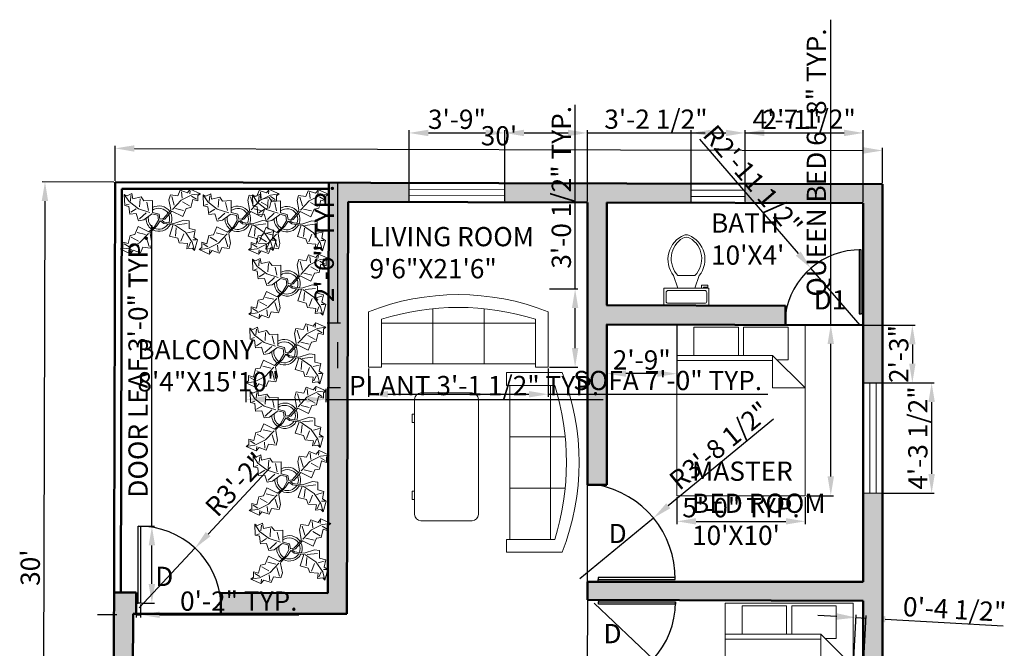
# Model space of a CAD drawing. Units: inches. Extents: x 16989 to 17950, y 7982 to 8536.
# Tile 5 of 5: x 17489 to 17950, y 8242 to 8536. Entities that reach past the tile are written whole.
import ezdxf

# ---------------------------------------------------------------- set-up
doc = ezdxf.new("R2010")
doc.units = ezdxf.units.IN
for name, color, linetype, lineweight in [('A-ANNO-DIMS', 2, 'Continuous', 18), ('A-ANNO-IDEN', 7, 'Continuous', 18), ('A-AREA-IDEN', 7, 'Continuous', 25), ('A-DOOR', 3, 'Continuous', 25), ('A-FLOR-FIXT', 9, 'Continuous', 18), ('A-FURN', 8, 'Continuous', 18), ('A-GLAZ', 4, 'Continuous', 18), ('A-WALL', 7, 'Continuous', 50), ('L-PLNT', 94, 'Continuous', 13)]:
    doc.layers.add(name, color=color, linetype=linetype, lineweight=lineweight)
doc.layers.add('A-WALL-PATT', color=177, linetype='Continuous', lineweight=13, true_color=0x293189)
doc.styles.get("Standard").update_dxf_attribs({"font": 'arial.ttf'})
doc.dimstyles.new('ISO-25', dxfattribs={"dimtxt": 9, "dimasz": 9, "dimexe": 1.25, "dimexo": 0.625, "dimtad": 1, "dimdec": 1, "dimrnd": 9, "dimlunit": 3, "dimtxsty": 'Standard', "dimcen": 2.5, "dimadec": 0, "dimazin": 0, "dimtfac": 1, "dimtdec": 1, "dimtmove": 0, "dimatfit": 3, "dimfxl": 1, "dimarcsym": 0})

# ---------------------------------------------------------------- blocks, each defined once
blk = doc.blocks.new('*D10')
at = {"layer": 'A-ANNO-DIMS', "color": 0, "lineweight": -2, "transparency": 16777216}
for p, q in [((17533.26, 8460.26), (17499.84, 8460.35)), ((17501.06, 8451.35), (17500.13, 8108.37)), ((17532.27, 8099.28), (17498.85, 8099.37))]:
    blk.add_line(p, q, dxfattribs=at)
at = {"layer": 'A-ANNO-DIMS', "color": 0, "transparency": 16777216}
for points in [[(17499.56, 8451.35), (17502.56, 8451.34), (17501.09, 8460.35)], [(17498.63, 8108.37), (17501.63, 8108.36), (17500.1, 8099.37)]]:
    blk.add_solid(points, dxfattribs=at)
at = {"layer": 'Defpoints', "color": 0, "transparency": 16777216}
for p in [(17533.88, 8460.26), (17500.1, 8099.37), (17532.9, 8099.28)]:
    blk.add_point(p, dxfattribs=at)
at = {"layer": 'A-ANNO-DIMS', "color": 0, "transparency": 16777216, "insert": (17495.37, 8279.87), "char_height": 9, "attachment_point": 5, "rotation": 89.8438}
blk.add_mtext("30'", dxfattribs=at)
blk = doc.blocks.new('*D11')
at = {"layer": 'A-ANNO-DIMS', "color": 0, "lineweight": -2, "transparency": 16777216}
for p, q in [((17533.88, 8460.88), (17533.93, 8477.23)), ((17542.93, 8475.95), (17883.94, 8475.02)), ((17892.9, 8459.9), (17892.94, 8476.25))]:
    blk.add_line(p, q, dxfattribs=at)
at = {"layer": 'A-ANNO-DIMS', "color": 0, "transparency": 16777216}
for points in [[(17542.93, 8477.45), (17542.92, 8474.45), (17533.93, 8475.98)], [(17883.95, 8476.52), (17883.94, 8473.52), (17892.94, 8475)]]:
    blk.add_solid(points, dxfattribs=at)
at = {"layer": 'Defpoints', "color": 0, "transparency": 16777216}
for p in [(17892.94, 8475), (17533.88, 8460.26), (17892.9, 8459.28)]:
    blk.add_point(p, dxfattribs=at)
at = {"layer": 'A-ANNO-DIMS', "color": 0, "transparency": 16777216, "insert": (17713.45, 8480.71), "char_height": 9, "attachment_point": 5, "rotation": 359.8438}
blk.add_mtext("30'", dxfattribs=at)
blk = doc.blocks.new('Plant - Rubber or Philodendron')
for p, q in [((13.3837, 12.301), (14.68, 13.9039)), ((14.68, 13.9039), (19.3848, 11.8146)), ((-16.2005, 11.4774), (-13.9899, 8.1064)), ((-16.2005, 11.4774), (-14.8639, 10.7964)), ((-16.0159, 6.3329), (-16.2005, 11.4774)), ((-14.8639, 10.7964), (-12.6195, 11.8975)), ((-13.3174, 8.325), (-13.0735, 11.0065)), ((-12.6195, 11.8975), (-12.1909, 9.4345)), ((-12.1909, 9.4345), (-8.3829, 10.3)), ((-8.8369, 9.409), (-9.0894, 5.6095)), ((-8.3829, 10.3), (-7.0549, 8.501)), ((4.6914, 8.8812), (5.3859, 11.2828)), ((5.3859, 11.2828), (8.8871, 10.7908)), ((5.9878, 10.4842), (7.1971, 6.3869)), ((8.8871, 10.7908), (9.9809, 13.4933)), ((9.9809, 13.4933), (13.3837, 12.301)), ((15.3859, 11.3055), (10.3916, 8.7942)), ((10.5828, 12.6946), (10.8893, 9.7953)), ((14.5816, 13.2037), (14.3848, 11.8033)), ((15.2875, 10.6053), (17.5907, 9.2105)), ((19.3848, 11.8146), (15.3859, 11.3055)), ((19.3848, 11.8146), (18.1868, 10.9119)), ((18.1868, 10.9119), (18.1925, 8.4119)), ((-14.0069, 5.8704), (-16.0159, 6.3329)), ((-15.3434, 6.5514), (-13.9984, 6.9884)), ((-13.5868, 2.2894), (-14.0069, 5.8704)), ((-13.9899, 8.1064), (-9.5434, 4.7185)), ((-13.1329, 3.1804), (-10.6614, 4.727)), ((-9.5434, 4.7185), (-4.1917, 2.9888)), ((-7.0549, 8.501), (-3.0284, 8.6941)), ((-4.8529, 4.012), (-5.7184, 7.82)), ((-3.0284, 8.6941), (-3.0709, 3.1041)), ((4.6914, 8.8812), (5.5014, 4.4831)), ((10.3916, 8.7942), (6.2847, 4.4028)), ((7.7005, 4.8881), (11.5025, 3.9967)), ((14.2977, 6.1031), (10.9934, 7.9956)), ((12.7005, 4.8994), (11.1089, 1.1958)), ((14.8995, 5.3044), (12.7005, 4.8994)), ((15.7909, 9.1065), (14.8995, 5.3044)), ((18.1925, 8.4119), (15.7909, 9.1065)), ((-10.6784, 2.491), (-13.5868, 2.2894)), ((-9.5858, -0.8715), (-10.6784, 2.491)), ((-9.1318, 0.0195), (-5.9793, 2.9025)), ((-7.1228, -0.443), (-3.5248, 2.2131)), ((-3.5248, 2.2131), (-3.3011, 2.4355)), ((-3.3011, 2.4355), (-0.5306, 1.7947)), ((-3.0709, 3.1041), (0.0797, 2.3163)), ((-0.5306, 1.7947), (-0.2255, -0.5527)), ((-0.5306, 1.7947), (-0.5306, 1.7947)), ((0.0797, 2.3163), (0.4866, -0.031)), ((0.4866, -0.031), (2.1141, 0.2298)), ((2.1141, 0.2298), (5.4346, 3.9146)), ((6.1032, 3.6844), (2.8262, -0.031)), ((5.4346, 3.9146), (5.5014, 4.4831)), ((11.1089, 1.1958), (6.1032, 3.6844)), ((-11.3237, -7.2629), (-9.7321, -3.5593)), ((-9.7321, -3.5593), (-4.7264, -6.0479)), ((-7.1228, -0.443), (-9.5858, -0.8715)), ((-2.019, -3.6148), (-4.7264, -6.0479)), ((-4.0579, -6.2781), (-0.9375, -3.1608)), ((-2.019, -3.6148), (-0.2255, -0.5527)), ((-0.9375, -3.1608), (0.5883, -0.8135)), ((0.5883, -0.8135), (2.2447, -2.0916)), ((2.8262, -0.031), (1.3003, -0.5527)), ((1.3003, -0.5527), (2.4193, -1.4655)), ((2.2447, -2.0916), (6.7108, -2.6626)), ((2.4193, -1.4655), (6.895, -2.1175)), ((4.943, -7.9659), (6.7108, -2.6626)), ((11.6605, -0.5413), (6.895, -2.1175)), ((12.3677, -6.1981), (7.219, -2.6772)), ((8.125, -4.0768), (7.7715, -7.9659)), ((8.3544, -2.7453), (13.1973, -2.1704)), ((11.6605, -0.5413), (14.1354, -0.8948)), ((14.1354, -0.8948), (14.1354, -4.4304)), ((14.1354, -4.4304), (16.9638, -5.1375)), ((-14.4141, -11.4699), (-13.5228, -7.6679)), ((-13.5228, -7.6679), (-11.3237, -7.2629)), ((-12.921, -8.4665), (-9.6166, -10.359)), ((-6.3237, -7.2516), (-10.1257, -6.3602)), ((-9.0148, -11.1577), (-4.9047, -6.8122)), ((-4.611, -12.8477), (-5.8203, -8.7504)), ((-4.1246, -6.8466), (-4.0579, -6.2781)), ((-3.3146, -11.2447), (-4.1246, -6.8466)), ((8.8321, -9.0266), (4.943, -7.9659)), ((9.5392, -11.1479), (8.8321, -9.0266)), ((10.2463, -10.4408), (11.6605, -6.9053)), ((15.5496, -10.7943), (12.3677, -6.1981)), ((16.2567, -5.8446), (13.4283, -6.5517)), ((16.9638, -5.1375), (16.2567, -8.673)), ((16.2567, -8.673), (18.0245, -9.7337)), ((-18.008, -14.1781), (-16.8101, -13.2754)), ((-18.008, -14.1781), (-14.0091, -13.669)), ((-16.8157, -10.7754), (-14.4141, -11.4699)), ((-16.8101, -13.2754), (-16.8157, -10.7754)), ((-13.9107, -12.9688), (-16.2139, -11.574)), ((-14.0091, -13.669), (-9.0148, -11.1577)), ((-9.206, -15.0581), (-9.5126, -12.1588)), ((-7.5103, -13.1543), (-8.6042, -15.8568)), ((-4.0092, -13.6463), (-7.5103, -13.1543)), ((-3.3146, -11.2447), (-4.0092, -13.6463)), ((13.4283, -11.5015), (9.5392, -11.1479)), ((13.0748, -13.9763), (13.4283, -11.5015)), ((15.5496, -13.6228), (13.0748, -13.9763)), ((14.8425, -10.7943), (13.7819, -13.2692)), ((16.6103, -14.6834), (15.5496, -10.7943)), ((16.6103, -14.6834), (15.5496, -13.6228)), ((17.3174, -9.7337), (15.9032, -9.7337)), ((18.0245, -9.7337), (16.6103, -14.6834)), ((-13.3032, -16.2674), (-18.008, -14.1781)), ((-12.0069, -14.6645), (-13.3032, -16.2674)), ((-13.2048, -15.5672), (-13.008, -14.1668)), ((-8.6042, -15.8568), (-12.0069, -14.6645))]:
    blk.add_line(p, q)
for centre, radius, start, end in [((0, 0), 6.1275, 34.37569, 120.1028), ((-0.0601, -0.2075), 5.2461, 33.82192, 124.9414), ((0.0308, 0.1664), 6, 178.6147, 235.1169), ((0.0308, 0.1664), 5, 168.1647, 238.6725), ((-0.2664, 0.1682), 5.2775, 338.4094, 20.03007), ((-0.098, 0.1364), 6.1288, 341.2017, 26.09184), ((-0.0234, 0.3825), 6.1492, 242.5812, 331.2714), ((-0.1102, 0.4886), 5.2883, 247.3711, 327.472)]:
    blk.add_arc(centre, radius, start, end)
blk = doc.blocks.new('Sofa - Roundback 7 ft.')
for p, q in [((-12.00002, -32.4421), (-12.00003, -6.5971)), ((11.99997, -32.4421), (11.99998, -6.5971)), ((-36.000027, -34), (-36.000027, -11.4696)), ((-35.999844, -13.3819), (35.9998, -13.3819)), ((35.99998, -34), (35.99998, -11.4696)), ((-36.000027, -32.4421), (35.99998, -32.4421))]:
    blk.add_line(p, q)
for points in [[(-36.000027, -34), (-42.000027, -34), (-42.000027, -8)], [(41.99998, -8), (41.99998, -34), (35.99998, -34)]]:
    blk.add_lwpolyline(points)
for centre, radius, start, end in [((0, -114.25), 114.25, 68.43141, 111.5686), ((-0.00001, -127.1968), 121.1968, 72.72033, 107.2797)]:
    blk.add_arc(centre, radius, start, end)
blk = doc.blocks.new('Desk - 30 x 60 in.')
for p, q in [((-26.999995, 0), (26.999995, 0)), ((-29.999995, -27), (-29.999995, -3)), ((29.999995, -3), (29.999995, -27)), ((26.999995, -30), (-26.999995, -30)), ((-20.000005, -30), (-20.000005, -31)), ((-20.000005, -31), (-16.000005, -31)), ((-16.000005, -31), (-16.000005, -30)), ((15.999995, -31), (15.999995, -30)), ((19.999995, -31), (15.999995, -31)), ((19.999995, -30), (19.999995, -31))]:
    blk.add_line(p, q)
for centre, start, end in [((-26.499995, -3.5), 98.1301, 171.8699), ((26.499995, -3.5), 8.130102, 81.8699), ((-26.499995, -26.5), 188.1301, 261.8699), ((26.499995, -26.5), 278.1301, 351.8699)]:
    blk.add_arc(centre, 3.535534, start, end)
blk = doc.blocks.new('Toilet - top')
for p, q in [((9.5, -6), (9.5, -2)), ((-10, -8.5), (-8, -8.5)), ((-10, -9.5), (-10, -8.5)), ((-8, -8.5), (-8, -8)), ((-7, -8), (-7, -9.5)), ((-4, -8), (-6, -14)), ((4, -8), (6, -14)), ((-7, -9.5), (-10, -9.5)), ((4, -14), (-4, -14))]:
    blk.add_line(p, q)
blk.add_lwpolyline([(10.5, -8), (10.5, 0), (-10.5, 0), (-10.5, -8)], close=True)
for points in [[(-9.5, -2), (-9.5, -6)], [(8.5, -1), (-8.5, -1)], [(-8.5, -7), (8.5, -7)]]:
    blk.add_lwpolyline(points)
for centre, radius, start, end in [((-8.62, -1.88), 0.884, 81.8699, 188.1301), ((8.62, -1.88), 0.884, 351.8699, 98.1301), ((-8.62, -6.12), 0.884, 171.8699, 278.1301), ((8.62, -6.12), 0.884, 261.8699, 8.1301), ((3.52, -21.58), 12.17, 141.4691, 247.9714), ((4.2, -21.82), 11.33, 136.3677, 238.9468), ((-3.52, -21.58), 12.17, 292.0284, 38.5307), ((-4.2, -21.82), 11.33, 301.053, 43.6321), ((0, -27.88), 4, 245.7318, 294.2682), ((0, -29), 4, 254.8605, 285.1395)]:
    blk.add_arc(centre, radius, start, end)
blk = doc.blocks.new('Bed - Queen')
for p, q in [((0, -80.00003), (0, 0)), ((0, 0), (59.99999, 0)), ((59.99999, 0), (59.99999, -80.00003)), ((7.99999, -1.2), (28.79998, -1.2)), ((7.99999, -14.4), (7.99999, -1.2)), ((28.79998, -1.2), (28.79998, -14.4)), ((31.19999, -1.2), (51.99999, -1.2)), ((31.19999, -14.4), (31.19999, -1.2)), ((51.99999, -1.2), (51.99999, -16.4)), ((0, -14.4), (44.8, -14.4)), ((44.8, -16.8), (0, -16.8)), ((59.99999, -29.6), (44.8, -14.4)), ((44.8, -14.4), (44.8, -29.6)), ((51.99999, -16.4), (46.79936, -16.4)), ((44.8, -29.6), (59.99999, -29.6)), ((59.99999, -80.00003), (0, -80.00003))]:
    blk.add_line(p, q)
blk = doc.blocks.new('DOOR-LEAF-30IN')
for p, q in [((1, 0), (1, 30)), ((1, 30), (2, 30)), ((2, 30), (2, 0)), ((0, 0), (1, 0)), ((2, 0), (1, 0))]:
    blk.add_line(p, q)
blk = doc.blocks.new('DOOR-LEAF-36IN')
for p, q in [((1, 0), (1, 36)), ((1, 36), (2, 36)), ((2, 36), (2, 0)), ((0, 0), (1, 0)), ((2, 0), (1, 0))]:
    blk.add_line(p, q)
blk = doc.blocks.new('*D15')
at = {"layer": 'A-ANNO-DIMS', "color": 0, "lineweight": -2, "transparency": 16777216}
for p, q in [((17595.1, 8363.58), (17595.1, 8357.35)), ((17632.49, 8363.58), (17632.49, 8357.35)), ((17604.1, 8358.6), (17623.49, 8358.6)), ((17632.49, 8358.6), (17762.15, 8358.6))]:
    blk.add_line(p, q, dxfattribs=at)
at = {"layer": 'A-ANNO-DIMS', "color": 0, "transparency": 16777216}
for points in [[(17604.1, 8360.1), (17604.1, 8357.1), (17595.1, 8358.6)], [(17623.49, 8360.1), (17623.49, 8357.1), (17632.49, 8358.6)]]:
    blk.add_solid(points, dxfattribs=at)
at = {"layer": 'Defpoints', "color": 0, "transparency": 16777216}
for p in [(17595.1, 8364.21), (17632.49, 8364.21), (17632.49, 8358.6)]:
    blk.add_point(p, dxfattribs=at)
at = {"layer": 'A-ANNO-DIMS', "color": 0, "transparency": 16777216, "insert": (17701.82, 8363.88), "char_height": 9, "attachment_point": 5}
blk.add_mtext('PLANT 3\'-1 1/2" TYP.', dxfattribs=at)
blk = doc.blocks.new('*D16')
at = {"layer": 'A-ANNO-DIMS', "color": 0, "lineweight": -2, "transparency": 16777216}
for p, q in [((17638.1, 8394.38), (17638.1, 8459.64)), ((17633.12, 8394.38), (17639.35, 8394.38)), ((17638.1, 8373.21), (17638.1, 8385.38)), ((17633.12, 8364.21), (17639.35, 8364.21))]:
    blk.add_line(p, q, dxfattribs=at)
at = {"layer": 'A-ANNO-DIMS', "color": 0, "transparency": 16777216}
for points in [[(17636.6, 8385.38), (17639.6, 8385.38), (17638.1, 8394.38)], [(17636.6, 8373.21), (17639.6, 8373.21), (17638.1, 8364.21)]]:
    blk.add_solid(points, dxfattribs=at)
at = {"layer": 'Defpoints', "color": 0, "transparency": 16777216}
for p in [(17632.49, 8394.38), (17638.1, 8394.38), (17632.49, 8364.21)]:
    blk.add_point(p, dxfattribs=at)
at = {"layer": 'A-ANNO-DIMS', "color": 0, "transparency": 16777216, "insert": (17632.88, 8431.51), "char_height": 9, "attachment_point": 5, "rotation": 90}
blk.add_mtext('2\'-6" TYP.', dxfattribs=at)
blk = doc.blocks.new('*D19')
at = {"layer": 'A-ANNO-DIMS', "color": 0, "lineweight": -2, "transparency": 16777216}
for p, q in [((17652.47, 8372.96), (17652.47, 8359.73)), ((17736.47, 8372.96), (17736.47, 8359.73)), ((17661.47, 8360.98), (17727.47, 8360.98)), ((17736.47, 8360.98), (17839.26, 8360.98))]:
    blk.add_line(p, q, dxfattribs=at)
at = {"layer": 'A-ANNO-DIMS', "color": 0, "transparency": 16777216}
for points in [[(17661.47, 8362.48), (17661.47, 8359.48), (17652.47, 8360.98)], [(17727.47, 8362.48), (17727.47, 8359.48), (17736.47, 8360.98)]]:
    blk.add_solid(points, dxfattribs=at)
at = {"layer": 'Defpoints', "color": 0, "transparency": 16777216}
for p in [(17652.47, 8373.58), (17736.47, 8373.58), (17736.47, 8360.98)]:
    blk.add_point(p, dxfattribs=at)
at = {"layer": 'A-ANNO-DIMS', "color": 0, "transparency": 16777216, "insert": (17792.37, 8366.26), "char_height": 9, "attachment_point": 5}
blk.add_mtext('SOFA 7\'-0" TYP.', dxfattribs=at)
blk = doc.blocks.new('*D20')
at = {"layer": 'A-ANNO-DIMS', "color": 0, "lineweight": -2, "transparency": 16777216}
for p, q in [((17749.07, 8410.25), (17749.07, 8496.32)), ((17737.1, 8410.25), (17750.32, 8410.25)), ((17749.07, 8382.58), (17749.07, 8401.25)), ((17737.1, 8373.58), (17750.32, 8373.58))]:
    blk.add_line(p, q, dxfattribs=at)
at = {"layer": 'A-ANNO-DIMS', "color": 0, "transparency": 16777216}
for points in [[(17747.57, 8401.25), (17750.57, 8401.25), (17749.07, 8410.25)], [(17747.57, 8382.58), (17750.57, 8382.58), (17749.07, 8373.58)]]:
    blk.add_solid(points, dxfattribs=at)
at = {"layer": 'Defpoints', "color": 0, "transparency": 16777216}
for p in [(17736.47, 8410.25), (17749.07, 8410.25), (17736.47, 8373.58)]:
    blk.add_point(p, dxfattribs=at)
at = {"layer": 'A-ANNO-DIMS', "color": 0, "transparency": 16777216, "insert": (17743.79, 8457.78), "char_height": 9, "attachment_point": 5, "rotation": 90}
blk.add_mtext('3\'-0 1/2" TYP.', dxfattribs=at)
blk = doc.blocks.new('*D21')
at = {"layer": 'A-ANNO-DIMS', "color": 0, "lineweight": -2, "transparency": 16777216}
for p, q in [((17868.67, 8393.54), (17868.67, 8536.18)), ((17857.29, 8393.54), (17869.92, 8393.54)), ((17868.67, 8322.54), (17868.67, 8384.54)), ((17857.29, 8313.54), (17869.92, 8313.54))]:
    blk.add_line(p, q, dxfattribs=at)
at = {"layer": 'A-ANNO-DIMS', "color": 0, "transparency": 16777216}
for points in [[(17867.17, 8384.54), (17870.17, 8384.54), (17868.67, 8393.54)], [(17867.17, 8322.54), (17870.17, 8322.54), (17868.67, 8313.54)]]:
    blk.add_solid(points, dxfattribs=at)
at = {"layer": 'Defpoints', "color": 0, "transparency": 16777216}
for p in [(17856.67, 8393.54), (17868.67, 8393.54), (17856.67, 8313.54)]:
    blk.add_point(p, dxfattribs=at)
at = {"layer": 'A-ANNO-DIMS', "color": 0, "transparency": 16777216, "insert": (17863.11, 8469.36), "char_height": 9, "attachment_point": 5, "rotation": 90}
blk.add_mtext('QUEEN BED 6\'-8" TYP.', dxfattribs=at)
blk = doc.blocks.new('*D22')
at = {"layer": 'A-ANNO-DIMS', "color": 0, "lineweight": -2, "transparency": 16777216}
for p, q in [((17796.67, 8312.92), (17796.67, 8300.29)), ((17856.67, 8312.92), (17856.67, 8300.29)), ((17805.67, 8301.54), (17847.67, 8301.54))]:
    blk.add_line(p, q, dxfattribs=at)
at = {"layer": 'A-ANNO-DIMS', "color": 0, "transparency": 16777216}
for points in [[(17805.67, 8303.04), (17805.67, 8300.04), (17796.67, 8301.54)], [(17847.67, 8303.04), (17847.67, 8300.04), (17856.67, 8301.54)]]:
    blk.add_solid(points, dxfattribs=at)
at = {"layer": 'Defpoints', "color": 0, "transparency": 16777216}
for p in [(17796.67, 8313.54), (17856.67, 8313.54), (17856.67, 8301.54)]:
    blk.add_point(p, dxfattribs=at)
at = {"layer": 'A-ANNO-DIMS', "color": 0, "transparency": 16777216, "insert": (17826.67, 8306.76), "char_height": 9, "attachment_point": 5}
blk.add_mtext('5\'-0" TYP.', dxfattribs=at)
blk = doc.blocks.new('*D25')
at = {"layer": 'A-ANNO-DIMS', "color": 0, "lineweight": -2, "transparency": 16777216}
for p, q in [((17551.09, 8299.24), (17551.09, 8440.05)), ((17546.31, 8299.24), (17552.34, 8299.24)), ((17551.09, 8272.24), (17551.09, 8290.24)), ((17546.31, 8263.24), (17552.34, 8263.24))]:
    blk.add_line(p, q, dxfattribs=at)
at = {"layer": 'A-ANNO-DIMS', "color": 0, "transparency": 16777216}
for points in [[(17549.59, 8290.24), (17552.59, 8290.24), (17551.09, 8299.24)], [(17549.59, 8272.24), (17552.59, 8272.24), (17551.09, 8263.24)]]:
    blk.add_solid(points, dxfattribs=at)
at = {"layer": 'Defpoints', "color": 0, "transparency": 16777216}
for p in [(17545.69, 8299.24), (17551.09, 8299.24), (17545.69, 8263.24)]:
    blk.add_point(p, dxfattribs=at)
at = {"layer": 'A-ANNO-DIMS', "color": 0, "transparency": 16777216, "insert": (17545.8, 8374.15), "char_height": 9, "attachment_point": 5, "rotation": 90}
blk.add_mtext('DOOR LEAF 3\'-0" TYP.', dxfattribs=at)
blk = doc.blocks.new('*D26')
at = {"layer": 'A-ANNO-DIMS', "color": 0, "lineweight": -2, "transparency": 16777216}
for p, q in [((17543.69, 8262.62), (17543.69, 8256.59)), ((17545.69, 8262.62), (17545.69, 8256.59)), ((17534.69, 8257.84), (17525.69, 8257.84)), ((17543.69, 8257.84), (17545.69, 8257.84)), ((17554.69, 8257.84), (17619.79, 8257.84))]:
    blk.add_line(p, q, dxfattribs=at)
at = {"layer": 'A-ANNO-DIMS', "color": 0, "transparency": 16777216}
for points in [[(17534.69, 8259.34), (17534.69, 8256.34), (17543.69, 8257.84)], [(17554.69, 8259.34), (17554.69, 8256.34), (17545.69, 8257.84)]]:
    blk.add_solid(points, dxfattribs=at)
at = {"layer": 'Defpoints', "color": 0, "transparency": 16777216}
for p in [(17543.69, 8263.24), (17545.69, 8263.24), (17545.69, 8257.84)]:
    blk.add_point(p, dxfattribs=at)
at = {"layer": 'A-ANNO-DIMS', "color": 0, "transparency": 16777216, "insert": (17591.74, 8263.06), "char_height": 9, "attachment_point": 5}
blk.add_mtext('0\'-2" TYP.', dxfattribs=at)
blk = doc.blocks.new('*D51')
at = {"layer": 'A-ANNO-DIMS', "color": 0, "lineweight": -2, "transparency": 16777216}
for p, q in [((17716.18, 8451.39), (17716.18, 8484.46)), ((17754.82, 8451.28), (17754.82, 8484.46)), ((17725.18, 8483.21), (17745.82, 8483.21)), ((17754.82, 8483.21), (17809.96, 8483.21))]:
    blk.add_line(p, q, dxfattribs=at)
at = {"layer": 'A-ANNO-DIMS', "color": 0, "transparency": 16777216}
for points in [[(17725.18, 8484.71), (17725.18, 8481.71), (17716.18, 8483.21)], [(17745.82, 8484.71), (17745.82, 8481.71), (17754.82, 8483.21)]]:
    blk.add_solid(points, dxfattribs=at)
at = {"layer": 'Defpoints', "color": 0, "transparency": 16777216}
for p in [(17754.82, 8483.21), (17716.18, 8450.76), (17754.82, 8450.66)]:
    blk.add_point(p, dxfattribs=at)
at = {"layer": 'A-ANNO-DIMS', "color": 0, "transparency": 16777216, "insert": (17786.89, 8488.49), "char_height": 9, "attachment_point": 5}
blk.add_mtext('3\'-2 1/2"', dxfattribs=at)
blk = doc.blocks.new('*D52')
at = {"layer": 'A-ANNO-DIMS', "color": 0, "lineweight": -2, "transparency": 16777216}
for p, q in [((17671.43, 8451.51), (17671.43, 8484.46)), ((17716.18, 8451.39), (17716.18, 8484.46)), ((17680.43, 8483.21), (17707.18, 8483.21))]:
    blk.add_line(p, q, dxfattribs=at)
at = {"layer": 'A-ANNO-DIMS', "color": 0, "transparency": 16777216}
for points in [[(17680.43, 8484.71), (17680.43, 8481.71), (17671.43, 8483.21)], [(17707.18, 8484.71), (17707.18, 8481.71), (17716.18, 8483.21)]]:
    blk.add_solid(points, dxfattribs=at)
at = {"layer": 'Defpoints', "color": 0, "transparency": 16777216}
for p in [(17716.18, 8483.21), (17671.43, 8450.88), (17716.18, 8450.76)]:
    blk.add_point(p, dxfattribs=at)
at = {"layer": 'A-ANNO-DIMS', "color": 0, "transparency": 16777216, "insert": (17693.8, 8488.43), "char_height": 9, "attachment_point": 5}
blk.add_mtext('3\'-9"', dxfattribs=at)
blk = doc.blocks.new('*D53')
at = {"layer": 'A-ANNO-DIMS', "color": 0, "lineweight": -2, "transparency": 16777216}
for p, q in [((17828.62, 8451.08), (17828.62, 8484.46)), ((17883.9, 8450.93), (17883.9, 8484.46)), ((17837.62, 8483.21), (17874.9, 8483.21))]:
    blk.add_line(p, q, dxfattribs=at)
at = {"layer": 'A-ANNO-DIMS', "color": 0, "transparency": 16777216}
for points in [[(17837.62, 8484.71), (17837.62, 8481.71), (17828.62, 8483.21)], [(17874.9, 8484.71), (17874.9, 8481.71), (17883.9, 8483.21)]]:
    blk.add_solid(points, dxfattribs=at)
at = {"layer": 'Defpoints', "color": 0, "transparency": 16777216}
for p in [(17883.9, 8483.21), (17828.62, 8450.45), (17883.9, 8450.3)]:
    blk.add_point(p, dxfattribs=at)
at = {"layer": 'A-ANNO-DIMS', "color": 0, "transparency": 16777216, "insert": (17856.26, 8488.49), "char_height": 9, "attachment_point": 5}
blk.add_mtext('4\'-7 1/2"', dxfattribs=at)
blk = doc.blocks.new('*D54')
at = {"layer": 'A-ANNO-DIMS', "color": 0, "lineweight": -2, "transparency": 16777216}
for p, q in [((17803.38, 8451.15), (17803.38, 8484.46)), ((17828.62, 8451.08), (17828.62, 8484.46)), ((17812.38, 8483.21), (17819.62, 8483.21)), ((17828.62, 8483.21), (17862.95, 8483.21))]:
    blk.add_line(p, q, dxfattribs=at)
at = {"layer": 'A-ANNO-DIMS', "color": 0, "transparency": 16777216}
for points in [[(17812.38, 8484.71), (17812.38, 8481.71), (17803.38, 8483.21)], [(17819.62, 8484.71), (17819.62, 8481.71), (17828.62, 8483.21)]]:
    blk.add_solid(points, dxfattribs=at)
at = {"layer": 'Defpoints', "color": 0, "transparency": 16777216}
for p in [(17828.62, 8483.21), (17803.38, 8450.52), (17828.62, 8450.45)]:
    blk.add_point(p, dxfattribs=at)
at = {"layer": 'A-ANNO-DIMS', "color": 0, "transparency": 16777216, "insert": (17850.29, 8488.35), "char_height": 9, "attachment_point": 5}
blk.add_mtext('2\'-1"', dxfattribs=at)
blk = doc.blocks.new('*D55')
at = {"layer": 'A-ANNO-DIMS', "color": 0, "lineweight": -2, "transparency": 16777216}
for p, q in [((17884.52, 8393.3), (17908.1, 8393.3)), ((17906.85, 8384.3), (17906.85, 8375.33)), ((17884.52, 8366.33), (17908.1, 8366.33))]:
    blk.add_line(p, q, dxfattribs=at)
at = {"layer": 'A-ANNO-DIMS', "color": 0, "transparency": 16777216}
for points in [[(17905.35, 8384.3), (17908.35, 8384.3), (17906.85, 8393.3)], [(17905.35, 8375.33), (17908.35, 8375.33), (17906.85, 8366.33)]]:
    blk.add_solid(points, dxfattribs=at)
at = {"layer": 'Defpoints', "color": 0, "transparency": 16777216}
for p in [(17883.9, 8393.3), (17883.9, 8366.33), (17906.85, 8366.33)]:
    blk.add_point(p, dxfattribs=at)
at = {"layer": 'A-ANNO-DIMS', "color": 0, "transparency": 16777216, "insert": (17901.63, 8379.82), "char_height": 9, "attachment_point": 5, "rotation": 90}
blk.add_mtext('2\'-3"', dxfattribs=at)
blk = doc.blocks.new('*D56')
at = {"layer": 'A-ANNO-DIMS', "color": 0, "lineweight": -2, "transparency": 16777216}
for p, q in [((17893.52, 8366.33), (17917.1, 8366.33)), ((17915.85, 8357.33), (17915.85, 8323.71)), ((17893.52, 8314.71), (17917.1, 8314.71))]:
    blk.add_line(p, q, dxfattribs=at)
at = {"layer": 'A-ANNO-DIMS', "color": 0, "transparency": 16777216}
for points in [[(17914.35, 8357.33), (17917.35, 8357.33), (17915.85, 8366.33)], [(17914.35, 8323.71), (17917.35, 8323.71), (17915.85, 8314.71)]]:
    blk.add_solid(points, dxfattribs=at)
at = {"layer": 'Defpoints', "color": 0, "transparency": 16777216}
for p in [(17892.9, 8366.33), (17892.9, 8314.71), (17915.85, 8314.71)]:
    blk.add_point(p, dxfattribs=at)
at = {"layer": 'A-ANNO-DIMS', "color": 0, "transparency": 16777216, "insert": (17910.57, 8340.52), "char_height": 9, "attachment_point": 5, "rotation": 90}
blk.add_mtext('4\'-3 1/2"', dxfattribs=at)
blk = doc.blocks.new('*D70')
at = {"layer": 'A-ANNO-DIMS', "color": 0, "lineweight": -2, "transparency": 16777216}
for p, q in [((17763.9, 8393.01), (17763.84, 8369.43)), ((17796.66, 8392.92), (17796.6, 8369.34)), ((17787.6, 8370.62), (17772.84, 8370.66))]:
    blk.add_line(p, q, dxfattribs=at)
at = {"layer": 'A-ANNO-DIMS', "color": 0, "transparency": 16777216}
for points in [[(17772.85, 8372.16), (17772.84, 8369.16), (17763.84, 8370.68)], [(17787.61, 8372.12), (17787.6, 8369.12), (17796.6, 8370.59)]]:
    blk.add_solid(points, dxfattribs=at)
at = {"layer": 'Defpoints', "color": 0, "transparency": 16777216}
for p in [(17763.9, 8393.63), (17796.67, 8393.54), (17763.84, 8370.68)]:
    blk.add_point(p, dxfattribs=at)
at = {"layer": 'A-ANNO-DIMS', "color": 0, "transparency": 16777216, "insert": (17780.24, 8375.86), "char_height": 9, "attachment_point": 5, "rotation": 359.844}
blk.add_mtext('2\'-9"', dxfattribs=at)
blk = doc.blocks.new('*D71')
at = {"layer": 'A-ANNO-DIMS', "color": 0, "lineweight": -2, "transparency": 16777216}
for p, q in [((17871.53, 8257.03), (17862.55, 8257.54)), ((17879.26, 8234.23), (17880.59, 8257.77)), ((17880.52, 8256.52), (17885.19, 8256.26)), ((17883.93, 8233.97), (17885.27, 8257.51)), ((17894.18, 8255.75), (17949.24, 8252.63))]:
    blk.add_line(p, q, dxfattribs=at)
at = {"layer": 'A-ANNO-DIMS', "color": 0, "transparency": 16777216}
for points in [[(17871.62, 8258.53), (17871.45, 8255.53), (17880.52, 8256.52)], [(17894.27, 8257.25), (17894.1, 8254.25), (17885.19, 8256.26)]]:
    blk.add_solid(points, dxfattribs=at)
at = {"layer": 'Defpoints', "color": 0, "transparency": 16777216}
for p in [(17885.19, 8256.26), (17879.22, 8233.61), (17883.9, 8233.34)]:
    blk.add_point(p, dxfattribs=at)
at = {"layer": 'A-ANNO-DIMS', "color": 0, "transparency": 16777216, "insert": (17926.5, 8259.21), "char_height": 9, "attachment_point": 5, "rotation": 356.7619}
blk.add_mtext('0\'-4 1/2"', dxfattribs=at)
blk = doc.blocks.new('*D77')
at = {"layer": 'A-ANNO-DIMS', "color": 0, "lineweight": -2, "transparency": 16777216}
for p, q in [((17841.89, 8349.35), (17792.66, 8308.82)), ((17751.31, 8274.78), (17785.72, 8303.1))]:
    blk.add_line(p, q, dxfattribs=at)
at = {"layer": 'A-ANNO-DIMS', "color": 0, "transparency": 16777216}
blk.add_solid([(17791.71, 8309.98), (17793.62, 8307.66), (17785.72, 8303.1)], dxfattribs=at)
at = {"layer": 'Defpoints', "color": 0, "transparency": 16777216}
for p in [(17785.72, 8303.1), (17751.31, 8274.78)]:
    blk.add_point(p, dxfattribs=at)
at = {"layer": 'A-ANNO-DIMS', "color": 0, "transparency": 16777216, "insert": (17817.39, 8336.02), "char_height": 9, "attachment_point": 5, "rotation": 39.4655}
blk.add_mtext('R3\'-8 1/2"', dxfattribs=at)
blk = doc.blocks.new('*D78')
at = {"layer": 'A-ANNO-DIMS', "color": 0, "lineweight": -2, "transparency": 16777216}
for p, q in [((17606.57, 8326.86), (17577.39, 8295.56)), ((17545.19, 8261.01), (17571.26, 8288.98))]:
    blk.add_line(p, q, dxfattribs=at)
at = {"layer": 'A-ANNO-DIMS', "color": 0, "transparency": 16777216}
blk.add_solid([(17576.3, 8296.58), (17578.49, 8294.54), (17571.26, 8288.98)], dxfattribs=at)
at = {"layer": 'Defpoints', "color": 0, "transparency": 16777216}
for p in [(17571.26, 8288.98), (17545.19, 8261.01)]:
    blk.add_point(p, dxfattribs=at)
at = {"layer": 'A-ANNO-DIMS', "color": 0, "transparency": 16777216, "insert": (17591.23, 8318.06), "char_height": 9, "attachment_point": 5, "rotation": 47.0084}
blk.add_mtext('R3\'-2"', dxfattribs=at)
blk = doc.blocks.new('*D79')
at = {"layer": 'A-ANNO-DIMS', "color": 0, "lineweight": -2, "transparency": 16777216}
for p, q in [((17757.95, 8263.31), (17785.52, 8237.11)), ((17823.06, 8201.44), (17792.04, 8230.91))]:
    blk.add_line(p, q, dxfattribs=at)
at = {"layer": 'A-ANNO-DIMS', "color": 0, "transparency": 16777216}
blk.add_solid([(17793.08, 8232), (17791.01, 8229.83), (17785.52, 8237.11)], dxfattribs=at)
at = {"layer": 'Defpoints', "color": 0, "transparency": 16777216}
for p in [(17757.95, 8263.31), (17785.52, 8237.11)]:
    blk.add_point(p, dxfattribs=at)
at = {"layer": 'A-ANNO-DIMS', "color": 0, "transparency": 16777216, "insert": (17814.41, 8216.86), "char_height": 9, "attachment_point": 5, "rotation": 316.4577}
blk.add_mtext('R3\'-2"', dxfattribs=at)
blk = doc.blocks.new('*D81')
at = {"layer": 'A-ANNO-DIMS', "color": 0, "lineweight": -2, "transparency": 16777216}
for p, q in [((17807.21, 8480.32), (17853.46, 8426.77)), ((17882.4, 8393.27), (17859.34, 8419.96))]:
    blk.add_line(p, q, dxfattribs=at)
at = {"layer": 'A-ANNO-DIMS', "color": 0, "transparency": 16777216}
blk.add_solid([(17854.6, 8427.75), (17852.33, 8425.79), (17859.34, 8419.96)], dxfattribs=at)
at = {"layer": 'Defpoints', "color": 0, "transparency": 16777216}
for p in [(17859.34, 8419.96), (17882.4, 8393.27)]:
    blk.add_point(p, dxfattribs=at)
at = {"layer": 'A-ANNO-DIMS', "color": 0, "transparency": 16777216, "insert": (17831.39, 8460.4), "char_height": 9, "attachment_point": 5, "rotation": 310.817}
blk.add_mtext('R2\'-11 1/2"', dxfattribs=at)

msp = doc.modelspace()

# ---------------------------------------------------------------- hatches: boundary and pattern name
at = {"layer": 'A-WALL-PATT'}
h = msp.add_hatch(color=256, dxfattribs=at)
h.dxf.hatch_style = 1
h.paths.add_polyline_path([(17542.33, 8258.28), (17543.69, 8258.28), (17543.69, 8268.21), (17533.36, 8268.23), (17532.9, 8099.28), (17806.25, 8099.28), (17806.25, 8108.28), (17763.9, 8108.28), (17763.9, 8147.63), (17846.7, 8147.44), (17846.72, 8156.44), (17763.9, 8156.63), (17763.9, 8225.31), (17754.87, 8225.31), (17754.88, 8192.66), (17625.57, 8192.96), (17622.88, 8192.97), (17622.88, 8183.96), (17625.57, 8183.96), (17754.88, 8183.99), (17754.9, 8108.28), (17541.92, 8108.28)])
h.paths.add_polyline_path([(17642.86, 8450.96), (17671.43, 8450.88), (17671.45, 8459.88), (17633.88, 8459.99), (17633.79, 8424.48), (17633.8, 8424.47), (17633.79, 8424.46), (17633.54, 8332.73), (17633.99, 8332.52), (17633.53, 8332.18), (17633.45, 8301.15), (17634.83, 8300.54), (17633.63, 8299.64), (17633.64, 8297.14), (17633.44, 8297.2), (17633.39, 8279.04), (17633.47, 8278.99), (17633.39, 8278.71), (17633.36, 8267.96), (17583.36, 8268.1), (17583.36, 8258.28), (17642.33, 8258.28)])
h.paths.add_polyline_path([(17763.9, 8450.63), (17803.38, 8450.52), (17803.4, 8459.52), (17716.21, 8459.76), (17716.18, 8450.76), (17754.82, 8450.66), (17754.85, 8318.6), (17763.9, 8318.6), (17763.9, 8393.63), (17796.67, 8393.54), (17847.42, 8393.54), (17847.45, 8402.4), (17801.15, 8402.53), (17790.65, 8402.53), (17790.65, 8402.56), (17763.9, 8402.63)])
h.paths.add_polyline_path([(17892.9, 8459.28), (17828.65, 8459.45), (17828.62, 8450.45), (17883.9, 8450.3), (17883.9, 8366.33), (17892.9, 8366.33)])
h.paths.add_polyline_path([(17892.9, 8314.71), (17883.9, 8314.71), (17883.9, 8273.3), (17754.86, 8273.28), (17754.86, 8264.83), (17883.9, 8264.35), (17883.9, 8233.34), (17892.9, 8233.34)])
h.paths.add_polyline_path([(17892.9, 8188.92), (17883.9, 8188.92), (17883.9, 8108.28), (17830.51, 8108.28), (17830.51, 8099.28), (17892.9, 8099.28)])

# ---------------------------------------------------------------- linework, layer by layer
at = {"layer": 'A-DOOR'}
for p, q in [((17754.86, 8273.28), (17754.85, 8318.6)), ((17754.87, 8231.11), (17755, 8264.83))]:
    msp.add_line(p, q, dxfattribs=at)
for centre, radius, start, end in [((17882.4, 8393.27), 35.27, 89.1877, 172.4476), ((17751.31, 8274.78), 44.56, 359.3571, 79.5739), ((17545.19, 8261.01), 38.24, 3.2664, 90.7493), ((17757.95, 8263.31), 38.03, 272.1614, 0.7533)]:
    msp.add_arc(centre, radius, start, end, dxfattribs=at)
at = {"layer": 'A-GLAZ'}
for p, q in [((17671.45, 8459.88), (17671.43, 8450.88)), ((17671.44, 8456.88), (17716.2, 8456.76)), ((17716.21, 8459.76), (17716.18, 8450.76)), ((17803.4, 8459.52), (17803.38, 8450.52)), ((17828.65, 8459.45), (17828.62, 8450.45)), ((17671.44, 8453.88), (17716.19, 8453.76)), ((17803.39, 8453.52), (17828.63, 8453.45)), ((17803.4, 8456.52), (17828.64, 8456.45)), ((17892.9, 8366.33), (17883.9, 8366.33)), ((17886.9, 8366.33), (17886.9, 8314.71)), ((17889.9, 8366.33), (17889.9, 8314.71)), ((17892.9, 8314.71), (17883.9, 8314.71))]:
    msp.add_line(p, q, dxfattribs=at)
at = {"layer": 'A-WALL'}
for p, q in [((17532.9, 8099.28), (17533.88, 8460.26)), ((17533.88, 8460.26), (17892.9, 8459.28)), ((17537.1, 8457.1), (17536.59, 8268.23)), ((17633.87, 8457.1), (17537.1, 8457.1)), ((17633.36, 8267.96), (17633.88, 8459.99)), ((17892.9, 8459.28), (17892.9, 8099.28)), ((17642.33, 8258.28), (17642.86, 8450.96)), ((17642.86, 8450.96), (17754.82, 8450.66)), ((17754.82, 8450.66), (17754.85, 8318.6)), ((17763.9, 8450.63), (17763.9, 8402.63)), ((17763.9, 8450.63), (17883.9, 8450.3)), ((17883.9, 8450.3), (17883.9, 8273.3)), ((17763.77, 8402.63), (17847.45, 8402.4)), ((17847.45, 8402.4), (17847.42, 8393.4)), ((17763.75, 8393.63), (17883.9, 8393.3)), ((17763.9, 8393.63), (17763.9, 8318.6)), ((17763.9, 8318.6), (17754.85, 8318.6)), ((17754.86, 8273.28), (17883.9, 8273.3)), ((17754.86, 8273.28), (17754.86, 8264.83)), ((17543.69, 8268.21), (17533.36, 8268.23)), ((17543.69, 8268.21), (17543.69, 8258.28)), ((17633.36, 8267.96), (17583.36, 8268.1)), ((17583.36, 8268.1), (17583.36, 8258.28)), ((17754.86, 8264.83), (17883.9, 8264.35)), ((17883.9, 8264.35), (17883.9, 8108.28)), ((17541.92, 8108.28), (17542.33, 8258.28)), ((17642.33, 8258.28), (17542.33, 8258.28))]:
    msp.add_line(p, q, dxfattribs=at)

# ---------------------------------------------------------------- block references
at = {"layer": 'A-DOOR', "extrusion": (0, 0, -1), "zscale": -1}
msp.add_blockref('DOOR-LEAF-30IN', (-17883.9, 8398.53), dxfattribs=at)
at = {"layer": 'A-DOOR'}
msp.add_blockref('DOOR-LEAF-36IN', (17543.69, 8263.24), dxfattribs=at)
at = {"layer": 'A-DOOR', "extrusion": (0, 0, -1), "zscale": -1, "rotation": 89.99999999999984}
msp.add_blockref('DOOR-LEAF-36IN', (-17759.87, 8273.28), dxfattribs=at)
at = {"layer": 'A-DOOR', "rotation": 269.9999999999998}
msp.add_blockref('DOOR-LEAF-36IN', (17759.98, 8264.81), dxfattribs=at)
at = {"layer": 'A-FLOR-FIXT', "rotation": 180}
msp.add_blockref('Toilet - top', (17801.15, 8402.53), dxfattribs=at)
at = {"layer": 'A-FURN'}
for name, p in [('Sofa - Roundback 7 ft.', (17694.47, 8407.58)), ('Bed - Queen', (17796.67, 8393.54)), ('Bed - Queen', (17819.22, 8263.21))]:
    msp.add_blockref(name, p, dxfattribs=at)
at = {"layer": 'A-FURN', "rotation": 270}
for name, p in [('Sofa - Roundback 7 ft.', (17751, 8329.09)), ('Desk - 30 x 60 in.', (17703.88, 8331.72))]:
    msp.add_blockref(name, p, dxfattribs=at)
at = {"layer": 'L-PLNT'}
for p in [(17554.39, 8442.97), (17591.25, 8442.85), (17614.29, 8442.71), (17614.41, 8412.66), (17613.11, 8380.47), (17613.21, 8350.76), (17614.61, 8320.71), (17615.44, 8288.73)]:
    msp.add_blockref('Plant - Rubber or Philodendron', p, dxfattribs=at)

# ---------------------------------------------------------------- texts
at = {"layer": 'A-ANNO-IDEN', "char_height": 9, "attachment_point": 1}
for s, insert in [('D1', (17860.73, 8409.63)), ('D', (17764.77, 8300.34)), ('D', (17552.67, 8280.29)), ('D', (17762.34, 8253.52))]:
    msp.add_mtext_dynamic_manual_height_columns(s, width=18.2953, gutter_width=12.5, heights=[0], dxfattribs=dict(at, insert=insert))
at = {"layer": 'A-AREA-IDEN', "char_height": 9, "attachment_point": 1}
for s, width, insert in [("BATH\\P10'X4'", 78.1764, (17812.65, 8445.57)), ('LIVING ROOM\\P9\'6"X21\'6"', 116.5024, (17652.88, 8439.21)), ('BALCONY\\P8\'4"X15\'10"', 78.1764, (17544.33, 8386.34)), ("MASTER\\PBED ROOM\\P10'X10'", 78.1764, (17803.77, 8329.5))]:
    msp.add_mtext_dynamic_manual_height_columns(s, width=width, gutter_width=12.5, heights=[0], dxfattribs=dict(at, insert=insert))

# ---------------------------------------------------------------- dimensions: what is measured, and where the dimension line sits
at = {"layer": 'A-ANNO-DIMS'}
for base, p1, p2, text, picture, middle in [((17868.67, 8393.54), (17856.67, 8313.54), (17856.67, 8393.54), 'QUEEN BED <> TYP.', '*D21', (17863.11, 8469.36)), ((17749.07, 8410.25), (17736.47, 8373.58), (17736.47, 8410.25), '<> TYP.', '*D20', (17743.79, 8457.78)), ((17638.1, 8394.38), (17632.49, 8364.21), (17632.49, 8394.38), '<> TYP.', '*D16', (17632.88, 8431.51)), ((17551.09, 8299.24), (17545.69, 8263.24), (17545.69, 8299.24), 'DOOR LEAF <> TYP.', '*D25', (17545.8, 8374.15))]:
    dim = msp.add_linear_dim(base=base, p1=p1, p2=p2, angle=90, text=text, dimstyle='ISO-25', override={"dimdec": 1, "dimlfac": 1, "dimrnd": 0, "dimzin": 1, "dimdsep": 46, "dimlunit": 4, "dimfrac": 2}, dxfattribs=at)
    dim.commit()
    dim.dimension.update_dxf_attribs({"geometry": picture, "text_midpoint": middle})
for base, p1, p2, picture, middle in [((17754.82, 8483.21), (17716.18, 8450.76), (17754.82, 8450.66), '*D51', (17786.89, 8488.49)), ((17883.9, 8483.21), (17828.62, 8450.45), (17883.9, 8450.3), '*D53', (17856.26, 8488.49)), ((17716.1819, 8483.208), (17671.4279, 8450.8828), (17716.1819, 8450.7608), '*D52', (17693.8049, 8488.4312)), ((17828.62, 8483.21), (17803.38, 8450.52), (17828.62, 8450.45), '*D54', (17850.29, 8488.35))]:
    dim = msp.add_linear_dim(base=base, p1=p1, p2=p2, dimstyle='ISO-25', override={"dimdec": 1, "dimlfac": 1, "dimrnd": 0, "dimzin": 1, "dimdsep": 46, "dimlunit": 4, "dimfrac": 2}, dxfattribs=at)
    dim.commit()
    dim.dimension.update_dxf_attribs({"geometry": picture, "text_midpoint": middle})
for p2, distance, picture, middle in [((17892.9, 8459.28), 15.72, '*D11', (17713.45, 8480.71)), ((17532.9, 8099.28), -32.8, '*D10', (17495.37, 8279.87))]:
    dim = msp.add_aligned_dim(p1=(17533.88, 8460.26), p2=p2, distance=distance, dimstyle='ISO-25', override={"dimclrd": 0, "dimclre": 0, "dimclrt": 0}, dxfattribs=at)
    dim.commit()
    dim.dimension.update_dxf_attribs({"geometry": picture, "text_midpoint": middle})
for center, mpoint, picture, middle in [((17882.4, 8393.27), (17859.34, 8419.96), '*D81', (17831.39, 8460.4)), ((17751.31, 8274.78), (17785.72, 8303.1), '*D77', (17817.39, 8336.02)), ((17545.19, 8261.01), (17571.26, 8288.98), '*D78', (17591.23, 8318.06)), ((17757.95, 8263.31), (17785.52, 8237.11), '*D79', (17814.41, 8216.86))]:
    dim = msp.add_radius_dim(center=center, mpoint=mpoint, dimstyle='ISO-25', override={"dimdec": 1, "dimlfac": 1, "dimrnd": 0, "dimzin": 1, "dimdsep": 46, "dimlunit": 4, "dimfrac": 2}, dxfattribs=at)
    dim.commit()
    dim.dimension.update_dxf_attribs({"geometry": picture, "text_midpoint": middle})
for base, p1, p2, text, picture, middle in [((17632.49, 8358.6), (17595.1, 8364.21), (17632.49, 8364.21), 'PLANT <> TYP.', '*D15', (17701.82, 8363.88)), ((17736.47, 8360.98), (17652.47, 8373.58), (17736.47, 8373.58), 'SOFA <> TYP.', '*D19', (17792.37, 8366.26)), ((17856.67, 8301.54), (17796.67, 8313.54), (17856.67, 8313.54), '<> TYP.', '*D22', (17826.67, 8306.76)), ((17545.69, 8257.84), (17543.69, 8263.24), (17545.69, 8263.24), '<> TYP.', '*D26', (17591.74, 8263.06))]:
    dim = msp.add_linear_dim(base=base, p1=p1, p2=p2, text=text, dimstyle='ISO-25', override={"dimdec": 1, "dimlfac": 1, "dimrnd": 0, "dimzin": 1, "dimdsep": 46, "dimlunit": 4, "dimfrac": 2}, dxfattribs=at)
    dim.commit()
    dim.dimension.update_dxf_attribs({"geometry": picture, "text_midpoint": middle})
for base, p1, p2, angle, picture, middle in [((17763.84, 8370.68), (17796.67, 8393.54), (17763.9, 8393.63), 179.844, '*D70', (17780.24, 8375.86)), ((17906.85, 8366.33), (17883.9, 8393.3), (17883.9, 8366.33), 270, '*D55', (17901.63, 8379.82)), ((17915.85, 8314.71), (17892.9, 8366.33), (17892.9, 8314.71), 90, '*D56', (17910.57, 8340.52)), ((17885.19, 8256.26), (17879.22, 8233.61), (17883.9, 8233.34), 356.7619, '*D71', (17926.5, 8259.21))]:
    dim = msp.add_linear_dim(base=base, p1=p1, p2=p2, angle=angle, dimstyle='ISO-25', override={"dimdec": 1, "dimlfac": 1, "dimrnd": 0, "dimzin": 1, "dimdsep": 46, "dimlunit": 4, "dimfrac": 2}, dxfattribs=at)
    dim.commit()
    dim.dimension.update_dxf_attribs({"geometry": picture, "text_midpoint": middle})

doc.saveas('drawing.dxf')
